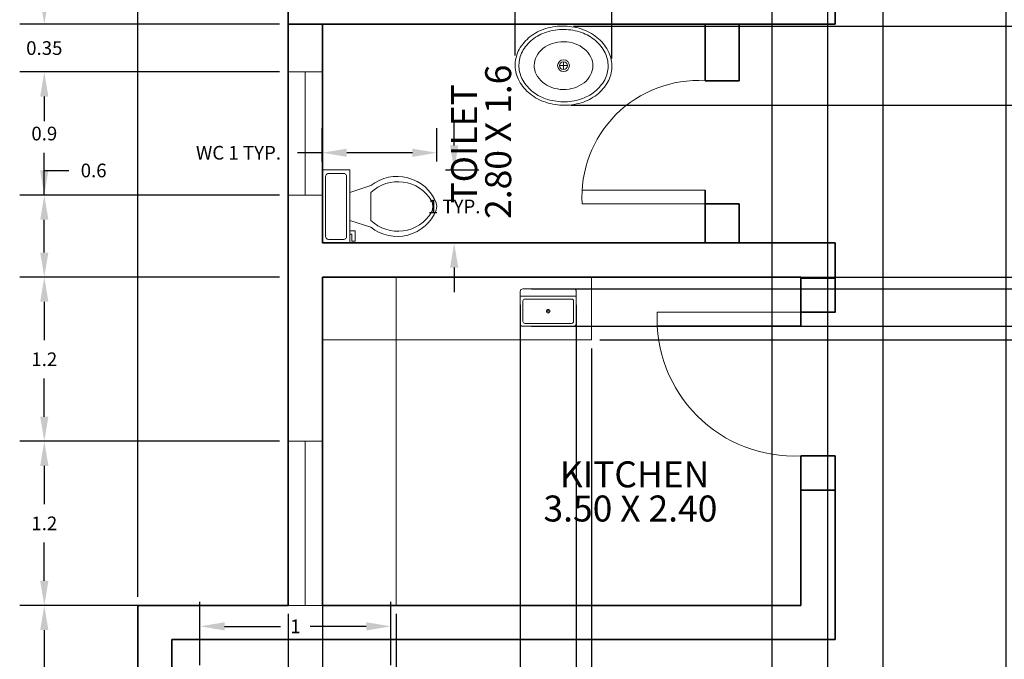
# Model space of a CAD drawing. Units: metres. Extents: x 180.3 to 196.1, y 135.7 to 166.1.
# Tile 3 of 5: x 180.3 to 187.5, y 156.1 to 160.8. Entities that reach past the tile are written whole.
import ezdxf

# ---------------------------------------------------------------- set-up
doc = ezdxf.new("R2010")
doc.units = ezdxf.units.M
doc.header["$MEASUREMENT"] = 0
for name, color, linetype, lineweight in [('A-ANNO-DIMS', 2, 'Continuous', 18), ('A-AREA-IDEN', 210, 'Continuous', 18), ('A-FLOR-CASE', 8, 'Continuous', 18), ('A-FLOR-FIXT', 9, 'Continuous', 18), ('A-GLAZ', 130, 'Continuous', 18), ('A-GLAZ-VENT', 170, 'Continuous', 18), ('dim', 70, 'Continuous', 15), ('door', 240, 'Continuous', 18), ('wall', 50, 'Continuous', 35)]:
    doc.layers.add(name, color=color, linetype=linetype, lineweight=lineweight)
doc.styles.get("Standard").update_dxf_attribs({"font": 'arial.ttf', "height": 0.1})
doc.dimstyles.get("Standard").update_dxf_attribs({"dimtxt": 0.18, "dimasz": 0.18, "dimexe": 0.18, "dimexo": 0.0625, "dimgap": 0.09, "dimtad": 0, "dimtih": 1, "dimtoh": 1, "dimdec": 4, "dimzin": 0, "dimdsep": 46, "dimtxsty": 'Standard', "dimcen": 0.09, "dimadec": 0, "dimazin": 0, "dimtfac": 1, "dimtdec": 4, "dimtofl": 0, "dimtmove": 0, "dimatfit": 3, "dimfxl": 1, "dimtolj": 1, "dimtzin": 0, "dimarcsym": 0})

# ---------------------------------------------------------------- blocks, each defined once
blk = doc.blocks.new('Sink - Oval top')
for p, q in [((-1, 0), (1, 0)), ((0, 1), (0, -1))]:
    blk.add_line(p, q)
for points in [[(-12.23, 0.39, 0.117634), (-11.46, -3.36, 0.104469), (-8.88, -6.8, 0.090016), (-5.08, -9.07, 0.08192), (-0.32, -10.02, 0.08192), (4.49, -9.38, 0.090016), (8.42, -7.36, 0.104469), (11.22, -4.09, 0.117634), (12.23, -0.39, 0.117634), (11.46, 3.36, 0.104469), (8.88, 6.8, 0.090016), (5.08, 9.07, 0.08192), (0.32, 10.02, 0.08192), (-4.49, 9.38, 0.090016), (-8.42, 7.36, 0.104469), (-11.22, 4.09, 0.117634)], [(-11.29, 0.16, 0.118622), (-10.52, -3.25, 0.104678), (-8.07, -6.36, 0.089562), (-4.54, -8.37, 0.081185), (-0.13, -9.15, 0.081185), (4.3, -8.49, 0.089562), (7.89, -6.58, 0.104678), (10.42, -3.55, 0.118622), (11.29, -0.16, 0.118622), (10.52, 3.25, 0.104678), (8.07, 6.36, 0.089562), (4.54, 8.37, 0.081185), (0.13, 9.15, 0.081185), (-4.3, 8.49, 0.089562), (-7.89, 6.58, 0.104678), (-10.42, 3.55, 0.118622)], [(-7.42, 0.08, 0.118283), (-6.91, -2.17, 0.104607), (-5.29, -4.21, 0.089718), (-2.97, -5.53, 0.081436), (-0.07, -6.04, 0.081436), (2.84, -5.59, 0.089718), (5.2, -4.33, 0.104607), (6.86, -2.32, 0.118283), (7.42, -0.08, 0.118283), (6.91, 2.17, 0.104607), (5.29, 4.21, 0.089718), (2.97, 5.53, 0.081436), (0.07, 6.04, 0.081436), (-2.84, 5.59, 0.089718), (-5.2, 4.33, 0.104607), (-6.86, 2.32, 0.118283)]]:
    blk.add_lwpolyline(points, format="xyb", close=True)
for radius in [1.5, 1]:
    blk.add_circle((0, 0), radius)
blk = doc.blocks.new('Toilet - top')
for p, q in [((9.5, -6), (9.5, -2)), ((-10, -8.5), (-8, -8.5)), ((-10, -9.5), (-10, -8.5)), ((-8, -8.5), (-8, -8)), ((-7, -8), (-7, -9.5)), ((-4, -8), (-6, -14)), ((4, -8), (6, -14)), ((-7, -9.5), (-10, -9.5)), ((4, -14), (-4, -14))]:
    blk.add_line(p, q)
blk.add_lwpolyline([(10.5, -8), (10.5, 0), (-10.5, 0), (-10.5, -8)], close=True)
for points in [[(-9.5, -2), (-9.5, -6)], [(8.5, -1), (-8.5, -1)], [(-8.5, -7), (8.5, -7)]]:
    blk.add_lwpolyline(points)
for centre, radius, start, end in [((-8.62, -1.88), 0.884, 81.8699, 188.1301), ((8.62, -1.88), 0.884, 351.8699, 98.1301), ((-8.62, -6.12), 0.884, 171.8699, 278.1301), ((8.62, -6.12), 0.884, 261.8699, 8.1301), ((3.52, -21.58), 12.17, 141.4691, 247.9714), ((4.2, -21.82), 11.33, 136.3677, 238.9468), ((-3.52, -21.58), 12.17, 292.0284, 38.5307), ((-4.2, -21.82), 11.33, 301.053, 43.6321), ((0, -27.88), 4, 245.7318, 294.2682), ((0, -29), 4, 254.8605, 285.1395)]:
    blk.add_arc(centre, radius, start, end)
blk = doc.blocks.new('Sink-single - 30 in top')
blk.add_line((-15, -3.999996), (15, -3.999996))
for points in [[(-13.5, 0), (13.5, 0)], [(-15, -18.499996), (-15, -1.5)], [(15, -1.5), (15, -18.499996)], [(-13.5, -17.499996), (-13.5, -6.499996)], [(-12.5, -5.499996), (12.5, -5.499996)], [(13.5, -6.499996), (13.5, -17.499996)], [(13.5, -19.999996), (-13.5, -19.999996)], [(12.5, -18.499996), (-12.5, -18.499996)]]:
    blk.add_lwpolyline(points)
for radius in [1, 0.5]:
    blk.add_circle((0, -11.999996), radius)
for centre, radius, start, end in [((-13.5, -1.5), 1.5, 90, 180), ((13.5, -1.5), 1.5, 0, 90), ((-12.5, -6.499996), 1, 90, 180), ((12.5, -6.499996), 1, 0, 90), ((-13.5, -18.499996), 1.5, 180, 270), ((-12.5, -17.499996), 1, 180, 270), ((12.5, -17.499996), 1, 270, 0), ((13.5, -18.499996), 1.5, 270, 0)]:
    blk.add_arc(centre, radius, start, end)
blk = doc.blocks.new('DOOR-1050')
for p, q in [((0.0004, -0.0001), (0.0004, 1.0499)), ((0.1004, -0.0001), (0.1004, 1.0499))]:
    blk.add_line(p, q)
blk.add_arc((0.0504, 0.0499), 1.0012, 357.13759, 92.86241)
blk = doc.blocks.new('DOOR-900')
for p, q in [((0.8013, -0.0001), (0.8013, 0.8999)), ((0.9013, -0.0001), (0.9013, 0.8999))]:
    blk.add_line(p, q)
blk.add_arc((0.8513, 0.0499), 0.8515, 86.63354, 183.36646)
blk = doc.blocks.new('WIN-1200')
for p, q in [((0.0003, 1.1999), (0.2503, 1.1999)), ((0.1253, -0.0001), (0.1253, 1.1999)), ((0.0003, -0.0001), (0.2503, -0.0001))]:
    blk.add_line(p, q)
blk = doc.blocks.new('VENT-900')
for p, q in [((0.0003, -0.0001), (0.0003, 0.2499)), ((0.9003, -0.0001), (0.9003, 0.2499)), ((0.9003, 0.1249), (0.0003, 0.1249))]:
    blk.add_line(p, q)
blk = doc.blocks.new('*D23')
at = {"layer": 'A-ANNO-DIMS', "color": 0, "lineweight": -2, "transparency": 16777216}
for p, q in [((182.5462, 159.744), (182.5462, 159.9874)), ((183.3856, 159.744), (183.3856, 159.9874)), ((182.5462, 159.8074), (182.3662, 159.8074)), ((183.2056, 159.8074), (182.7262, 159.8074))]:
    blk.add_line(p, q, dxfattribs=at)
at = {"layer": 'A-ANNO-DIMS', "color": 0, "transparency": 16777216}
for points in [[(182.7262, 159.8374), (182.7262, 159.7774), (182.5462, 159.8074)], [(183.2056, 159.8374), (183.2056, 159.7774), (183.3856, 159.8074)]]:
    blk.add_solid(points, dxfattribs=at)
at = {"layer": 'Defpoints', "color": 0, "transparency": 16777216}
for p in [(182.5462, 159.8074), (182.5462, 159.6815), (183.3856, 159.6815)]:
    blk.add_point(p, dxfattribs=at)
at = {"layer": 'A-ANNO-DIMS', "color": 0, "transparency": 16777216, "insert": (181.9338, 159.8074), "char_height": 0.1, "attachment_point": 5}
blk.add_mtext('\\A1;WC 1 TYP.', dxfattribs=at)
blk = doc.blocks.new('*D24')
at = {"layer": 'A-ANNO-DIMS', "color": 0, "lineweight": -2, "transparency": 16777216}
for p, q in [((183.5115, 159.8615), (183.5115, 160.0415)), ((183.4481, 159.6815), (183.6915, 159.6815)), ((183.4481, 159.1481), (183.6915, 159.1481)), ((183.5115, 158.9681), (183.5115, 158.7881))]:
    blk.add_line(p, q, dxfattribs=at)
at = {"layer": 'A-ANNO-DIMS', "color": 0, "transparency": 16777216}
for points in [[(183.4815, 159.8615), (183.5415, 159.8615), (183.5115, 159.6815)], [(183.4815, 158.9681), (183.5415, 158.9681), (183.5115, 159.1481)]]:
    blk.add_solid(points, dxfattribs=at)
at = {"layer": 'Defpoints', "color": 0, "transparency": 16777216}
for p in [(183.3856, 159.6815), (183.5115, 159.6815), (183.3856, 159.1481)]:
    blk.add_point(p, dxfattribs=at)
at = {"layer": 'A-ANNO-DIMS', "color": 0, "transparency": 16777216, "insert": (183.5115, 159.4148), "char_height": 0.1, "attachment_point": 5}
blk.add_mtext('\\A1;1 TYP.', dxfattribs=at)
blk = doc.blocks.new('*D26')
at = {"layer": 'A-ANNO-DIMS', "color": 0, "lineweight": -2, "transparency": 16777216}
for p, q in [((181.6518, 156.0609), (181.6518, 156.5251)), ((183.0488, 156.0609), (183.0488, 156.5251)), ((181.8318, 156.3451), (182.2419, 156.3451)), ((182.8688, 156.3451), (182.4587, 156.3451))]:
    blk.add_line(p, q, dxfattribs=at)
at = {"layer": 'A-ANNO-DIMS', "color": 0, "transparency": 16777216}
for points in [[(181.8318, 156.3751), (181.8318, 156.3151), (181.6518, 156.3451)], [(182.8688, 156.3751), (182.8688, 156.3151), (183.0488, 156.3451)]]:
    blk.add_solid(points, dxfattribs=at)
at = {"layer": 'Defpoints', "color": 0, "transparency": 16777216}
for p in [(183.0488, 156.3451), (181.6518, 155.9984), (183.0488, 155.9984)]:
    blk.add_point(p, dxfattribs=at)
at = {"layer": 'A-ANNO-DIMS', "color": 0, "transparency": 16777216, "insert": (182.3503, 156.3451), "char_height": 0.1, "attachment_point": 5}
blk.add_mtext('\\A1;1', dxfattribs=at)
blk = doc.blocks.new('*D33')
at = {"layer": 'A-ANNO-DIMS', "color": 0, "lineweight": -2, "transparency": 16777216}
for p, q in [((181.1973, 156.5604), (181.1973, 166.1117)), ((194.8473, 160.8104), (194.8473, 166.1117)), ((181.3773, 165.9317), (187.7679, 165.9317)), ((194.6673, 165.9317), (188.2767, 165.9317))]:
    blk.add_line(p, q, dxfattribs=at)
at = {"layer": 'A-ANNO-DIMS', "color": 0, "transparency": 16777216}
for points in [[(181.3773, 165.9617), (181.3773, 165.9017), (181.1973, 165.9317)], [(194.6673, 165.9617), (194.6673, 165.9017), (194.8473, 165.9317)]]:
    blk.add_solid(points, dxfattribs=at)
at = {"layer": 'Defpoints', "color": 0, "transparency": 16777216}
for p in [(194.8473, 165.9317), (194.8473, 160.7479), (181.1973, 156.4979)]:
    blk.add_point(p, dxfattribs=at)
at = {"layer": 'A-ANNO-DIMS', "color": 0, "transparency": 16777216, "insert": (188.0223, 165.9317), "char_height": 0.1, "attachment_point": 5}
blk.add_mtext('\\A1;13.65', dxfattribs=at)
blk = doc.blocks.new('*D35')
at = {"layer": 'A-ANNO-DIMS', "color": 0, "lineweight": -2, "transparency": 16777216}
for p, q in [((181.1973, 156.5604), (181.1973, 166.1117)), ((182.2973, 156.5604), (182.2973, 166.1117)), ((181.3773, 165.9317), (181.5807, 165.9317)), ((182.1173, 165.9317), (181.914, 165.9317))]:
    blk.add_line(p, q, dxfattribs=at)
at = {"layer": 'A-ANNO-DIMS', "color": 0, "transparency": 16777216}
for points in [[(181.3773, 165.9617), (181.3773, 165.9017), (181.1973, 165.9317)], [(182.1173, 165.9617), (182.1173, 165.9017), (182.2973, 165.9317)]]:
    blk.add_solid(points, dxfattribs=at)
at = {"layer": 'Defpoints', "color": 0, "transparency": 16777216}
for p in [(182.2973, 165.9317), (181.1973, 156.4979), (182.2973, 156.4979)]:
    blk.add_point(p, dxfattribs=at)
at = {"layer": 'A-ANNO-DIMS', "color": 0, "transparency": 16777216, "insert": (181.7473, 165.9317), "char_height": 0.1, "attachment_point": 5}
blk.add_mtext('\\A1;1.1', dxfattribs=at)
blk = doc.blocks.new('*D36')
at = {"layer": 'A-ANNO-DIMS', "color": 0, "lineweight": -2, "transparency": 16777216}
for p, q in [((181.1348, 156.4979), (180.3336, 156.4979)), ((180.5136, 156.3179), (180.5136, 154.2638)), ((180.5136, 151.9279), (180.5136, 153.982)), ((181.1348, 151.7479), (180.3336, 151.7479))]:
    blk.add_line(p, q, dxfattribs=at)
at = {"layer": 'A-ANNO-DIMS', "color": 0, "transparency": 16777216}
for points in [[(180.4836, 156.3179), (180.5436, 156.3179), (180.5136, 156.4979)], [(180.4836, 151.9279), (180.5436, 151.9279), (180.5136, 151.7479)]]:
    blk.add_solid(points, dxfattribs=at)
at = {"layer": 'Defpoints', "color": 0, "transparency": 16777216}
for p in [(180.5136, 156.4979), (181.1973, 156.4979), (181.1973, 151.7479)]:
    blk.add_point(p, dxfattribs=at)
at = {"layer": 'A-ANNO-DIMS', "color": 0, "transparency": 16777216, "insert": (180.5136, 154.1229), "char_height": 0.1, "attachment_point": 5}
blk.add_mtext('\\A1;4.75', dxfattribs=at)
blk = doc.blocks.new('*D38')
at = {"layer": 'A-ANNO-DIMS', "color": 0, "lineweight": -2, "transparency": 16777216}
for p, q in [((182.2348, 165.2479), (180.3336, 165.2479)), ((180.5136, 165.0679), (180.5136, 163.1388)), ((180.5136, 160.9279), (180.5136, 162.857)), ((182.2348, 160.7479), (180.3336, 160.7479))]:
    blk.add_line(p, q, dxfattribs=at)
at = {"layer": 'A-ANNO-DIMS', "color": 0, "transparency": 16777216}
for points in [[(180.4836, 165.0679), (180.5436, 165.0679), (180.5136, 165.2479)], [(180.4836, 160.9279), (180.5436, 160.9279), (180.5136, 160.7479)]]:
    blk.add_solid(points, dxfattribs=at)
at = {"layer": 'Defpoints', "color": 0, "transparency": 16777216}
for p in [(182.2973, 165.2479), (180.5136, 160.7479), (182.2973, 160.7479)]:
    blk.add_point(p, dxfattribs=at)
at = {"layer": 'A-ANNO-DIMS', "color": 0, "transparency": 16777216, "insert": (180.5136, 162.9979), "char_height": 0.1, "attachment_point": 5}
blk.add_mtext('\\A1;4.5', dxfattribs=at)
blk = doc.blocks.new('*D45')
at = {"layer": 'A-ANNO-DIMS', "color": 0, "lineweight": -2, "transparency": 16777216}
for p, q in [((182.2348, 157.6979), (180.3336, 157.6979)), ((180.5136, 157.5179), (180.5136, 157.2381)), ((180.5136, 156.6779), (180.5136, 156.9577)), ((182.2348, 156.4979), (180.3336, 156.4979))]:
    blk.add_line(p, q, dxfattribs=at)
at = {"layer": 'A-ANNO-DIMS', "color": 0, "transparency": 16777216}
for points in [[(180.4836, 157.5179), (180.5436, 157.5179), (180.5136, 157.6979)], [(180.4836, 156.6779), (180.5436, 156.6779), (180.5136, 156.4979)]]:
    blk.add_solid(points, dxfattribs=at)
at = {"layer": 'Defpoints', "color": 0, "transparency": 16777216}
for p in [(180.5136, 157.6979), (182.2973, 157.6979), (182.2973, 156.4979)]:
    blk.add_point(p, dxfattribs=at)
at = {"layer": 'A-ANNO-DIMS', "color": 0, "transparency": 16777216, "insert": (180.5136, 157.0979), "char_height": 0.1, "attachment_point": 5}
blk.add_mtext('\\A1;1.2', dxfattribs=at)
blk = doc.blocks.new('*D46')
at = {"layer": 'A-ANNO-DIMS', "color": 0, "lineweight": -2, "transparency": 16777216}
for p, q in [((182.2348, 158.8979), (180.3336, 158.8979)), ((180.5136, 158.7179), (180.5136, 158.4381)), ((180.5136, 157.8779), (180.5136, 158.1577)), ((182.2348, 157.6979), (180.3336, 157.6979))]:
    blk.add_line(p, q, dxfattribs=at)
at = {"layer": 'A-ANNO-DIMS', "color": 0, "transparency": 16777216}
for points in [[(180.4836, 158.7179), (180.5436, 158.7179), (180.5136, 158.8979)], [(180.4836, 157.8779), (180.5436, 157.8779), (180.5136, 157.6979)]]:
    blk.add_solid(points, dxfattribs=at)
at = {"layer": 'Defpoints', "color": 0, "transparency": 16777216}
for p in [(180.5136, 158.8979), (182.2973, 158.8979), (182.2973, 157.6979)]:
    blk.add_point(p, dxfattribs=at)
at = {"layer": 'A-ANNO-DIMS', "color": 0, "transparency": 16777216, "insert": (180.5136, 158.2979), "char_height": 0.1, "attachment_point": 5}
blk.add_mtext('\\A1;1.2', dxfattribs=at)
blk = doc.blocks.new('*D47')
at = {"layer": 'A-ANNO-DIMS', "color": 0, "lineweight": -2, "transparency": 16777216}
for p, q in [((180.5136, 159.4979), (180.5136, 159.6779)), ((180.5136, 159.6779), (180.6936, 159.6779)), ((182.2348, 159.4979), (180.3336, 159.4979)), ((180.5136, 159.0779), (180.5136, 159.3179)), ((182.2348, 158.8979), (180.3336, 158.8979))]:
    blk.add_line(p, q, dxfattribs=at)
at = {"layer": 'A-ANNO-DIMS', "color": 0, "transparency": 16777216}
for points in [[(180.4836, 159.3179), (180.5436, 159.3179), (180.5136, 159.4979)], [(180.4836, 159.0779), (180.5436, 159.0779), (180.5136, 158.8979)]]:
    blk.add_solid(points, dxfattribs=at)
at = {"layer": 'Defpoints', "color": 0, "transparency": 16777216}
for p in [(180.5136, 159.4979), (182.2973, 159.4979), (182.2973, 158.8979)]:
    blk.add_point(p, dxfattribs=at)
at = {"layer": 'A-ANNO-DIMS', "color": 0, "transparency": 16777216, "insert": (180.8746, 159.6779), "char_height": 0.1, "attachment_point": 5}
blk.add_mtext('\\A1;0.6', dxfattribs=at)
blk = doc.blocks.new('*D48')
at = {"layer": 'A-ANNO-DIMS', "color": 0, "lineweight": -2, "transparency": 16777216}
for p, q in [((182.2348, 160.3979), (180.3336, 160.3979)), ((180.5136, 160.2179), (180.5136, 160.089)), ((180.5136, 159.6779), (180.5136, 159.8068)), ((182.2348, 159.4979), (180.3336, 159.4979))]:
    blk.add_line(p, q, dxfattribs=at)
at = {"layer": 'A-ANNO-DIMS', "color": 0, "transparency": 16777216}
for points in [[(180.4836, 160.2179), (180.5436, 160.2179), (180.5136, 160.3979)], [(180.4836, 159.6779), (180.5436, 159.6779), (180.5136, 159.4979)]]:
    blk.add_solid(points, dxfattribs=at)
at = {"layer": 'Defpoints', "color": 0, "transparency": 16777216}
for p in [(180.5136, 160.3979), (182.2973, 160.3979), (182.2973, 159.4979)]:
    blk.add_point(p, dxfattribs=at)
at = {"layer": 'A-ANNO-DIMS', "color": 0, "transparency": 16777216, "insert": (180.5136, 159.9479), "char_height": 0.1, "attachment_point": 5}
blk.add_mtext('\\A1;0.9', dxfattribs=at)
blk = doc.blocks.new('*D49')
at = {"layer": 'A-ANNO-DIMS', "color": 0, "lineweight": -2, "transparency": 16777216}
for p, q in [((180.513585, 160.927902), (180.513585, 161.107902)), ((182.234835, 160.747902), (180.333585, 160.747902)), ((182.234835, 160.397902), (180.333585, 160.397902)), ((180.513585, 160.217902), (180.513585, 160.037902))]:
    blk.add_line(p, q, dxfattribs=at)
at = {"layer": 'A-ANNO-DIMS', "color": 0, "transparency": 16777216}
for points in [[(180.483585, 160.927902), (180.543585, 160.927902), (180.513585, 160.747902)], [(180.483585, 160.217902), (180.543585, 160.217902), (180.513585, 160.397902)]]:
    blk.add_solid(points, dxfattribs=at)
at = {"layer": 'Defpoints', "color": 0, "transparency": 16777216}
for p in [(180.513585, 160.747902), (182.297335, 160.747902), (182.297335, 160.397902)]:
    blk.add_point(p, dxfattribs=at)
at = {"layer": 'A-ANNO-DIMS', "color": 0, "transparency": 16777216, "insert": (180.513585, 160.572902), "char_height": 0.1, "attachment_point": 5}
blk.add_mtext('\\A1;0.35', dxfattribs=at)
blk = doc.blocks.new('*D50')
at = {"layer": 'A-ANNO-DIMS', "color": 0, "lineweight": -2, "transparency": 16777216}
for p, q in [((182.2973, 156.4354), (182.2973, 150.8842)), ((182.5473, 156.4354), (182.5473, 150.8842)), ((182.1173, 151.0642), (181.9373, 151.0642)), ((182.7273, 151.0642), (182.9073, 151.0642))]:
    blk.add_line(p, q, dxfattribs=at)
at = {"layer": 'A-ANNO-DIMS', "color": 0, "transparency": 16777216}
for points in [[(182.1173, 151.0942), (182.1173, 151.0342), (182.2973, 151.0642)], [(182.7273, 151.0942), (182.7273, 151.0342), (182.5473, 151.0642)]]:
    blk.add_solid(points, dxfattribs=at)
at = {"layer": 'Defpoints', "color": 0, "transparency": 16777216}
for p in [(182.2973, 156.4979), (182.5473, 156.4979), (182.5473, 151.0642)]:
    blk.add_point(p, dxfattribs=at)
at = {"layer": 'A-ANNO-DIMS', "color": 0, "transparency": 16777216, "insert": (183.1276, 151.0642), "char_height": 0.1, "attachment_point": 5}
blk.add_mtext('\\A1;0.25', dxfattribs=at)
blk = doc.blocks.new('*D51')
at = {"layer": 'A-ANNO-DIMS', "color": 0, "lineweight": -2, "transparency": 16777216}
for p, q in [((182.5473, 156.4354), (182.5473, 150.8842)), ((183.0878, 156.4354), (183.0878, 150.8842)), ((182.7273, 151.0642), (182.9078, 151.0642)), ((183.0878, 151.0642), (183.2678, 151.0642))]:
    blk.add_line(p, q, dxfattribs=at)
at = {"layer": 'A-ANNO-DIMS', "color": 0, "transparency": 16777216}
for points in [[(182.7273, 151.0942), (182.7273, 151.0342), (182.5473, 151.0642)], [(182.9078, 151.0942), (182.9078, 151.0342), (183.0878, 151.0642)]]:
    blk.add_solid(points, dxfattribs=at)
at = {"layer": 'Defpoints', "color": 0, "transparency": 16777216}
for p in [(182.5473, 156.4979), (183.0878, 156.4979), (183.0878, 151.0642)]:
    blk.add_point(p, dxfattribs=at)
at = {"layer": 'A-ANNO-DIMS', "color": 0, "transparency": 16777216, "insert": (183.4875, 151.0642), "char_height": 0.1, "attachment_point": 5}
blk.add_mtext('\\A1;0.54', dxfattribs=at)
blk = doc.blocks.new('*D52')
at = {"layer": 'A-ANNO-DIMS', "color": 0, "lineweight": -2, "transparency": 16777216}
for p, q in [((182.5473, 158.3772), (182.5473, 150.8842)), ((184.5151, 158.3772), (184.5151, 150.8842)), ((182.7273, 151.0642), (183.316, 151.0642)), ((184.3351, 151.0642), (183.7464, 151.0642))]:
    blk.add_line(p, q, dxfattribs=at)
at = {"layer": 'A-ANNO-DIMS', "color": 0, "transparency": 16777216}
for points in [[(182.7273, 151.0942), (182.7273, 151.0342), (182.5473, 151.0642)], [(184.3351, 151.0942), (184.3351, 151.0342), (184.5151, 151.0642)]]:
    blk.add_solid(points, dxfattribs=at)
at = {"layer": 'Defpoints', "color": 0, "transparency": 16777216}
for p in [(182.5473, 158.4397), (184.5151, 158.4397), (184.5151, 151.0642)]:
    blk.add_point(p, dxfattribs=at)
at = {"layer": 'A-ANNO-DIMS', "color": 0, "transparency": 16777216, "insert": (183.5312, 151.0642), "char_height": 0.1, "attachment_point": 5}
blk.add_mtext('\\A1;1.97', dxfattribs=at)
blk = doc.blocks.new('*D53')
at = {"layer": 'A-ANNO-DIMS', "color": 0, "lineweight": -2, "transparency": 16777216}
for p, q in [((195.531085, 159.077902), (195.531085, 159.257902)), ((184.57756, 158.897902), (195.711085, 158.897902)), ((184.57756, 158.43968), (195.711085, 158.43968)), ((195.531085, 158.25968), (195.531085, 158.07968))]:
    blk.add_line(p, q, dxfattribs=at)
at = {"layer": 'A-ANNO-DIMS', "color": 0, "transparency": 16777216}
for points in [[(195.501085, 159.077902), (195.561085, 159.077902), (195.531085, 158.897902)], [(195.501085, 158.25968), (195.561085, 158.25968), (195.531085, 158.43968)]]:
    blk.add_solid(points, dxfattribs=at)
at = {"layer": 'Defpoints', "color": 0, "transparency": 16777216}
for p in [(184.51506, 158.897902), (195.531085, 158.897902), (184.51506, 158.43968)]:
    blk.add_point(p, dxfattribs=at)
at = {"layer": 'A-ANNO-DIMS', "color": 0, "transparency": 16777216, "insert": (195.531085, 158.668791), "char_height": 0.1, "attachment_point": 5}
blk.add_mtext('\\A1;0.46', dxfattribs=at)
blk = doc.blocks.new('*D54')
at = {"layer": 'A-ANNO-DIMS', "color": 0, "lineweight": -2, "transparency": 16777216}
for p, q in [((186.6473, 162.1854), (186.6473, 150.8842)), ((187.5473, 162.1854), (187.5473, 150.8842)), ((186.8273, 151.0642), (187.3673, 151.0642)), ((187.5473, 151.0642), (187.7273, 151.0642))]:
    blk.add_line(p, q, dxfattribs=at)
at = {"layer": 'A-ANNO-DIMS', "color": 0, "transparency": 16777216}
for points in [[(186.8273, 151.0942), (186.8273, 151.0342), (186.6473, 151.0642)], [(187.3673, 151.0942), (187.3673, 151.0342), (187.5473, 151.0642)]]:
    blk.add_solid(points, dxfattribs=at)
at = {"layer": 'Defpoints', "color": 0, "transparency": 16777216}
for p in [(186.6473, 162.2479), (187.5473, 162.2479), (187.5473, 151.0642)]:
    blk.add_point(p, dxfattribs=at)
at = {"layer": 'A-ANNO-DIMS', "color": 0, "transparency": 16777216, "insert": (187.9085, 151.0642), "char_height": 0.1, "attachment_point": 5}
blk.add_mtext('\\A1;0.9', dxfattribs=at)
blk = doc.blocks.new('*D59')
at = {"layer": 'A-ANNO-DIMS', "color": 0, "lineweight": -2, "transparency": 16777216}
for p, q in [((183.958, 160.5181), (183.958, 166.1117)), ((184.6651, 160.4954), (184.6651, 166.1117)), ((184.138, 165.9317), (184.4851, 165.9317)), ((184.6651, 165.9317), (184.8451, 165.9317))]:
    blk.add_line(p, q, dxfattribs=at)
at = {"layer": 'A-ANNO-DIMS', "color": 0, "transparency": 16777216}
for points in [[(184.138, 165.9617), (184.138, 165.9017), (183.958, 165.9317)], [(184.4851, 165.9617), (184.4851, 165.9017), (184.6651, 165.9317)]]:
    blk.add_solid(points, dxfattribs=at)
at = {"layer": 'Defpoints', "color": 0, "transparency": 16777216}
for p in [(184.6651, 165.9317), (183.958, 160.4556), (184.6651, 160.4329)]:
    blk.add_point(p, dxfattribs=at)
at = {"layer": 'A-ANNO-DIMS', "color": 0, "transparency": 16777216, "insert": (185.1038, 165.9317), "char_height": 0.1, "attachment_point": 5}
blk.add_mtext('\\A1;0.707', dxfattribs=at)
blk = doc.blocks.new('*D60')
at = {"layer": 'A-ANNO-DIMS', "color": 0, "lineweight": -2, "transparency": 16777216}
for p, q in [((195.5311, 160.7337), (195.5311, 160.9137)), ((195.5311, 160.9137), (195.7111, 160.9137)), ((184.3834, 160.7337), (195.7111, 160.7337)), ((195.5311, 160.3348), (195.5311, 160.5537)), ((184.3647, 160.1548), (195.7111, 160.1548))]:
    blk.add_line(p, q, dxfattribs=at)
at = {"layer": 'A-ANNO-DIMS', "color": 0, "transparency": 16777216}
for points in [[(195.5011, 160.5537), (195.5611, 160.5537), (195.5311, 160.7337)], [(195.5011, 160.3348), (195.5611, 160.3348), (195.5311, 160.1548)]]:
    blk.add_solid(points, dxfattribs=at)
at = {"layer": 'Defpoints', "color": 0, "transparency": 16777216}
for p in [(184.3209, 160.7337), (195.5311, 160.7337), (184.3022, 160.1548)]:
    blk.add_point(p, dxfattribs=at)
at = {"layer": 'A-ANNO-DIMS', "color": 0, "transparency": 16777216, "insert": (195.9311, 160.9137), "char_height": 0.1, "attachment_point": 5}
blk.add_mtext('\\A1;0.58', dxfattribs=at)
blk = doc.blocks.new('*D61')
at = {"layer": 'A-ANNO-DIMS', "color": 0, "lineweight": -2, "transparency": 16777216}
for p, q in [((183.9941, 158.6956), (183.9941, 150.8842)), ((184.4049, 158.6956), (184.4049, 150.8842)), ((183.8141, 151.0642), (183.6341, 151.0642)), ((184.5849, 151.0642), (184.7649, 151.0642))]:
    blk.add_line(p, q, dxfattribs=at)
at = {"layer": 'A-ANNO-DIMS', "color": 0, "transparency": 16777216}
for points in [[(183.8141, 151.0942), (183.8141, 151.0342), (183.9941, 151.0642)], [(184.5849, 151.0942), (184.5849, 151.0342), (184.4049, 151.0642)]]:
    blk.add_solid(points, dxfattribs=at)
at = {"layer": 'Defpoints', "color": 0, "transparency": 16777216}
for p in [(183.9941, 158.7581), (184.4049, 158.7581), (184.4049, 151.0642)]:
    blk.add_point(p, dxfattribs=at)
at = {"layer": 'A-ANNO-DIMS', "color": 0, "transparency": 16777216, "insert": (184.9751, 151.0642), "char_height": 0.1, "attachment_point": 5}
blk.add_mtext('\\A1;0.41', dxfattribs=at)
blk = doc.blocks.new('*D62')
at = {"layer": 'A-ANNO-DIMS', "color": 0, "lineweight": -2, "transparency": 16777216}
for p, q in [((195.5311, 158.9929), (195.5311, 159.1729)), ((195.5311, 159.1729), (195.7111, 159.1729)), ((184.0771, 158.8129), (195.7111, 158.8129)), ((184.0771, 158.539), (195.7111, 158.539)), ((195.5311, 158.359), (195.5311, 158.179))]:
    blk.add_line(p, q, dxfattribs=at)
at = {"layer": 'A-ANNO-DIMS', "color": 0, "transparency": 16777216}
for points in [[(195.5011, 158.9929), (195.5611, 158.9929), (195.5311, 158.8129)], [(195.5011, 158.359), (195.5611, 158.359), (195.5311, 158.539)]]:
    blk.add_solid(points, dxfattribs=at)
at = {"layer": 'Defpoints', "color": 0, "transparency": 16777216}
for p in [(184.0146, 158.8129), (195.5311, 158.8129), (184.0146, 158.539)]:
    blk.add_point(p, dxfattribs=at)
at = {"layer": 'A-ANNO-DIMS', "color": 0, "transparency": 16777216, "insert": (195.931, 159.1729), "char_height": 0.1, "attachment_point": 5}
blk.add_mtext('\\A1;0.27', dxfattribs=at)
blk = doc.blocks.new('*D63')
at = {"layer": 'A-ANNO-DIMS', "color": 0, "lineweight": -2, "transparency": 16777216}
for p, q in [((185.8382, 153.8738), (185.8382, 166.1117)), ((186.2446, 153.8757), (186.2446, 166.1117)), ((185.6582, 165.9317), (185.4782, 165.9317)), ((186.4246, 165.9317), (186.6046, 165.9317))]:
    blk.add_line(p, q, dxfattribs=at)
at = {"layer": 'A-ANNO-DIMS', "color": 0, "transparency": 16777216}
for points in [[(185.6582, 165.9617), (185.6582, 165.9017), (185.8382, 165.9317)], [(186.4246, 165.9617), (186.4246, 165.9017), (186.2446, 165.9317)]]:
    blk.add_solid(points, dxfattribs=at)
at = {"layer": 'Defpoints', "color": 0, "transparency": 16777216}
for p in [(186.2446, 165.9317), (185.8382, 153.8113), (186.2446, 153.8132)]:
    blk.add_point(p, dxfattribs=at)
at = {"layer": 'A-ANNO-DIMS', "color": 0, "transparency": 16777216, "insert": (186.8148, 165.9317), "char_height": 0.1, "attachment_point": 5}
blk.add_mtext('\\A1;0.41', dxfattribs=at)

msp = doc.modelspace()

# ---------------------------------------------------------------- linework, layer by layer
at = {"layer": 'A-FLOR-CASE'}
for points in [[(182.5473, 158.8979), (183.0878, 158.8979), (183.0878, 156.4979), (182.5473, 156.4979)], [(182.5473, 158.8979), (184.5151, 158.8979), (184.5151, 158.4397), (182.5473, 158.4397)]]:
    msp.add_lwpolyline(points, close=True, dxfattribs=at)
at = {"layer": 'wall'}
for p, q in [((182.2973, 160.7479), (182.2973, 165.2479)), ((186.2973, 161.2479), (186.2973, 160.7479)), ((186.2973, 160.7479), (182.2973, 160.7479)), ((182.2973, 160.7479), (182.2973, 158.8979)), ((182.5473, 160.7479), (182.5473, 159.1479)), ((185.3473, 160.7479), (185.3473, 160.3344)), ((185.5973, 160.7479), (185.5973, 160.3344)), ((185.3473, 160.3344), (185.5973, 160.3344)), ((182.5473, 159.9479), (182.5473, 159.1479)), ((185.3473, 159.5344), (185.3473, 159.1479)), ((185.3473, 159.4344), (185.5973, 159.4344)), ((185.5973, 159.4344), (185.5973, 159.1479)), ((186.2973, 159.1479), (182.5473, 159.1479)), ((186.2973, 159.1479), (186.2973, 158.6415)), ((182.2973, 158.8979), (182.2973, 156.4979)), ((185.5973, 158.8979), (182.5473, 158.8979)), ((182.5473, 158.8979), (182.5473, 156.4979)), ((186.0473, 158.8979), (185.5973, 158.8979)), ((186.0473, 158.8979), (186.0473, 158.5415)), ((186.0473, 157.5915), (186.0473, 156.4979)), ((186.2973, 157.5915), (186.2973, 156.2479)), ((182.2973, 156.4979), (181.1973, 156.4979)), ((181.1973, 156.4979), (181.1973, 151.7479)), ((185.5973, 156.4979), (182.5473, 156.4979)), ((186.0473, 156.4979), (185.5973, 156.4979)), ((181.4473, 156.2479), (181.4473, 151.9979)), ((182.2973, 156.2479), (181.4473, 156.2479)), ((186.2973, 156.2479), (182.2973, 156.2479)), ((186.2973, 156.2479), (182.2973, 156.2479)), ((186.0473, 156.2479), (185.5973, 156.2479))]:
    msp.add_line(p, q, dxfattribs=at)
for points in [[(186.0473, 158.8915), (186.0473, 158.6415), (186.2973, 158.6415), (186.2973, 158.8915)], [(186.0473, 157.5915), (186.0473, 157.3415), (186.2973, 157.3415), (186.2973, 157.5915)]]:
    msp.add_lwpolyline(points, close=True, dxfattribs=at)

# ---------------------------------------------------------------- block references
at = {"layer": 'A-FLOR-FIXT'}
for name, p, xscale, yscale, zscale in [('Sink - Oval top', (184.3115, 160.4443), 0.0288968728577968, 0.0288968728577968, 0.0288968728577968), ('Sink-single - 30 in top', (184.1995, 158.8129), 0.0136929114071847, 0.0136929114071847, 0.0136929114071847)]:
    msp.add_blockref(name, p, dxfattribs=dict(at, xscale=xscale, yscale=yscale, zscale=zscale))
at = {"layer": 'A-FLOR-FIXT', "xscale": 0.0254, "yscale": 0.0254, "zscale": 0.0254, "rotation": 90}
msp.add_blockref('Toilet - top', (182.5462, 159.4148), dxfattribs=at)
at = {"layer": 'A-GLAZ', "rotation": 180}
msp.add_blockref('WIN-1200', (182.5477, 157.6978), dxfattribs=at)
at = {"layer": 'A-GLAZ-VENT', "rotation": 89.99999999999422}
msp.add_blockref('VENT-900', (182.5472, 159.4976), dxfattribs=at)
at = {"layer": 'door', "extrusion": (0, 0, -1), "zscale": -1}
for name, p, rotation in [('DOOR-900', (-185.3472, 160.3357), 269.9999999999964), ('DOOR-1050', (-186.0472, 158.6419), 269.9999999999969)]:
    msp.add_blockref(name, p, dxfattribs=dict(at, rotation=rotation))

# ---------------------------------------------------------------- texts
at = {"layer": 'A-AREA-IDEN', "insert": (183.4896, 159.436), "char_height": 0.19, "attachment_point": 1, "rotation": 90}
msp.add_mtext_dynamic_manual_height_columns('TOILET ', width=0.900113, gutter_width=1, heights=[0], dxfattribs=at)
at = {"layer": 'A-AREA-IDEN', "insert": (183.6337, 157.5511), "char_height": 0.19, "attachment_point": 1}
msp.add_mtext_dynamic_manual_height_columns('\\pxqc;KITCHEN', width=2.394331, gutter_width=1, heights=[0], dxfattribs=at)
at = {"layer": 'dim', "insert": (183.7385, 159.097), "char_height": 0.19, "attachment_point": 1, "rotation": 90}
msp.add_mtext_dynamic_manual_height_columns('\\pxqc;2.80 X 1.6', width=1.581155, gutter_width=1, heights=[0], dxfattribs=at)
at = {"layer": 'dim', "insert": (184.1649, 157.3015), "char_height": 0.19, "attachment_point": 1}
msp.add_mtext_dynamic_manual_height_columns('3.50 X 2.40 ', width=2.225522, gutter_width=1, heights=[0], dxfattribs=at)

# ---------------------------------------------------------------- dimensions: what is measured, and where the dimension line sits
at = {"layer": 'A-ANNO-DIMS'}
for base, p1, p2, override, picture, middle in [((194.8473, 165.9317), (181.1973, 156.4979), (194.8473, 160.7479), {"dimdec": 2, "dimlfac": 1, "dimrnd": 0, "dimzin": 0, "dimdsep": 46, "dimlunit": 2}, '*D33', (188.0223, 165.9317)), ((182.2973, 165.9317), (181.1973, 156.4979), (182.2973, 156.4979), {"dimdec": 1, "dimlfac": 1, "dimrnd": 0, "dimzin": 0, "dimdsep": 46, "dimlunit": 2}, '*D35', (181.7473, 165.9317)), ((184.6651, 165.9317), (183.958, 160.4556), (184.6651, 160.4329), {"dimdec": 3, "dimlfac": 1, "dimrnd": 0, "dimzin": 0, "dimdsep": 46, "dimlunit": 2}, '*D59', (185.1038, 165.9317)), ((186.2446, 165.9317), (185.8382, 153.8113), (186.2446, 153.8132), {"dimdec": 2, "dimlfac": 1, "dimrnd": 0, "dimzin": 0, "dimdsep": 46, "dimlunit": 2}, '*D63', (186.8148, 165.9317)), ((187.5473, 151.0642), (186.6473, 162.2479), (187.5473, 162.2479), {"dimdec": 1, "dimlfac": 1, "dimrnd": 0, "dimzin": 0, "dimdsep": 46, "dimlunit": 2}, '*D54', (187.9085, 151.0642)), ((184.4049, 151.0642), (183.9941, 158.7581), (184.4049, 158.7581), {"dimdec": 2, "dimlfac": 1, "dimrnd": 0, "dimzin": 0, "dimdsep": 46, "dimlunit": 2}, '*D61', (184.9751, 151.0642)), ((184.5151, 151.0642), (182.5473, 158.4397), (184.5151, 158.4397), {"dimdec": 2, "dimlfac": 1, "dimrnd": 0, "dimzin": 0, "dimdsep": 46, "dimlunit": 2}, '*D52', (183.5312, 151.0642)), ((183.0488, 156.3451), (181.6518, 155.9984), (183.0488, 155.9984), {"dimdec": 0, "dimlfac": 1, "dimrnd": 0, "dimzin": 0, "dimdsep": 46, "dimlunit": 2}, '*D26', (182.3503, 156.3451)), ((182.5473, 151.0642), (182.2973, 156.4979), (182.5473, 156.4979), {"dimdec": 2, "dimlfac": 1, "dimrnd": 0, "dimzin": 0, "dimdsep": 46, "dimlunit": 2}, '*D50', (183.1276, 151.0642)), ((183.0878, 151.0642), (182.5473, 156.4979), (183.0878, 156.4979), {"dimdec": 2, "dimlfac": 1, "dimrnd": 0, "dimzin": 0, "dimdsep": 46, "dimlunit": 2}, '*D51', (183.4875, 151.0642))]:
    dim = msp.add_linear_dim(base=base, p1=p1, p2=p2, dimstyle='Standard', override=override, dxfattribs=at)
    dim.commit()
    dim.dimension.update_dxf_attribs({"geometry": picture, "text_midpoint": middle})
for base, p1, p2, override, picture, middle in [((180.5136, 160.7479), (182.2973, 165.2479), (182.2973, 160.7479), {"dimdec": 1, "dimlfac": 1, "dimrnd": 0, "dimzin": 0, "dimdsep": 46, "dimlunit": 2}, '*D38', (180.5136, 162.9979)), ((180.5136, 160.7479), (182.2973, 160.3979), (182.2973, 160.7479), {"dimdec": 2, "dimlfac": 1, "dimrnd": 0, "dimzin": 0, "dimdsep": 46, "dimlunit": 2}, '*D49', (180.5136, 160.5729)), ((195.5311, 160.7337), (184.3022, 160.1548), (184.3209, 160.7337), {"dimdec": 2, "dimlfac": 1, "dimrnd": 0, "dimzin": 0, "dimdsep": 46, "dimlunit": 2}, '*D60', (195.9311, 160.9137)), ((180.5136, 160.3979), (182.2973, 159.4979), (182.2973, 160.3979), {"dimdec": 1, "dimlfac": 1, "dimrnd": 0, "dimzin": 0, "dimdsep": 46, "dimlunit": 2}, '*D48', (180.5136, 159.9479)), ((180.5136, 159.4979), (182.2973, 158.8979), (182.2973, 159.4979), {"dimdec": 1, "dimlfac": 1, "dimrnd": 0, "dimzin": 0, "dimdsep": 46, "dimlunit": 2}, '*D47', (180.8746, 159.6779)), ((195.5311, 158.8129), (184.0146, 158.539), (184.0146, 158.8129), {"dimdec": 2, "dimlfac": 1, "dimrnd": 0, "dimzin": 0, "dimdsep": 46, "dimlunit": 2}, '*D62', (195.931, 159.1729)), ((195.5311, 158.8979), (184.5151, 158.4397), (184.5151, 158.8979), {"dimdec": 2, "dimlfac": 1, "dimrnd": 0, "dimzin": 0, "dimdsep": 46, "dimlunit": 2}, '*D53', (195.5311, 158.6688)), ((180.5136, 158.8979), (182.2973, 157.6979), (182.2973, 158.8979), {"dimdec": 1, "dimlfac": 1, "dimrnd": 0, "dimzin": 0, "dimdsep": 46, "dimlunit": 2}, '*D46', (180.5136, 158.2979)), ((180.5136, 157.6979), (182.2973, 156.4979), (182.2973, 157.6979), {"dimdec": 1, "dimlfac": 1, "dimrnd": 0, "dimzin": 0, "dimdsep": 46, "dimlunit": 2}, '*D45', (180.5136, 157.0979)), ((180.5136, 156.4979), (181.1973, 151.7479), (181.1973, 156.4979), {"dimdec": 2, "dimlfac": 1, "dimrnd": 0, "dimzin": 0, "dimdsep": 46, "dimlunit": 2}, '*D36', (180.5136, 154.1229))]:
    dim = msp.add_linear_dim(base=base, p1=p1, p2=p2, angle=90, dimstyle='Standard', override=override, dxfattribs=at)
    dim.commit()
    dim.dimension.update_dxf_attribs({"geometry": picture, "text_midpoint": middle})
for base, p1, p2, angle, text, picture, middle in [((182.5462, 159.8074), (183.3856, 159.6815), (182.5462, 159.6815), 180, 'WC <> TYP.', '*D23', (181.9338, 159.8074)), ((183.5115, 159.6815), (183.3856, 159.1481), (183.3856, 159.6815), 90, '<> TYP.', '*D24', (183.5115, 159.4148))]:
    dim = msp.add_linear_dim(base=base, p1=p1, p2=p2, angle=angle, text=text, dimstyle='Standard', override={"dimdec": 0, "dimlfac": 1, "dimrnd": 0, "dimzin": 0, "dimdsep": 46, "dimlunit": 2}, dxfattribs=at)
    dim.commit()
    dim.dimension.update_dxf_attribs({"geometry": picture, "text_midpoint": middle})

doc.saveas('drawing.dxf')
